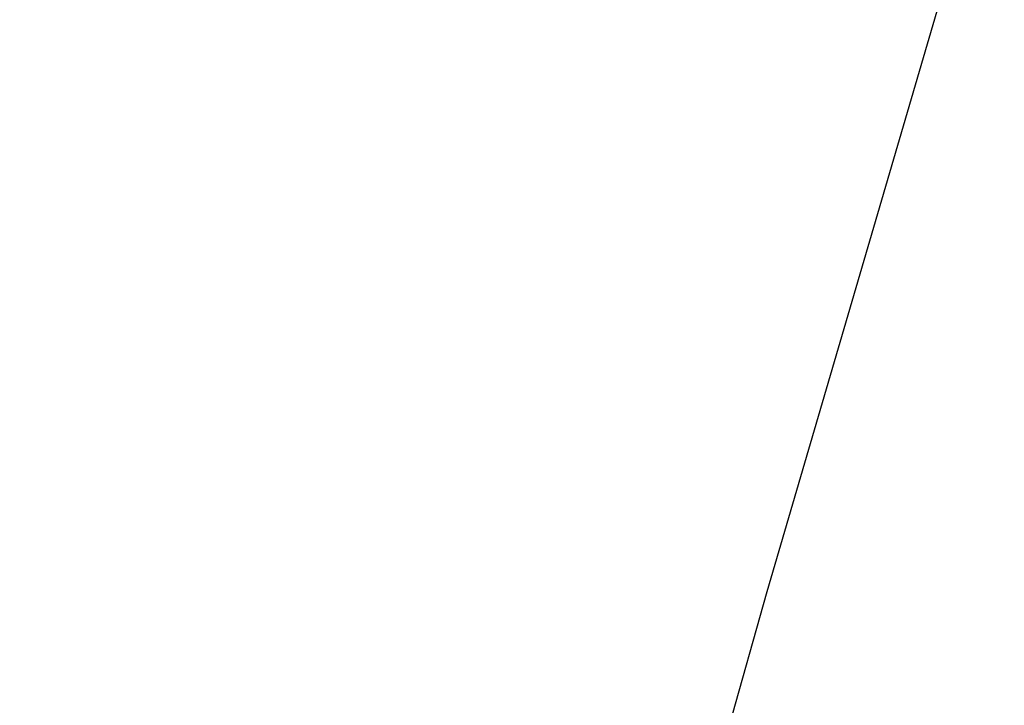
# Model space of a CAD drawing. Units: inches. Extents: x 3590 to 5167, y 65 to 1917.
# Tile 90 of 100: x 5052.5773 to 5052.8768, y 1788.6144 to 1788.8231. Entities that reach past the tile are written whole.
import ezdxf

# ---------------------------------------------------------------- set-up
doc = ezdxf.new("R2010")
doc.units = ezdxf.units.IN
for name, color, linetype, lineweight in [('A-ANNO-DIMS', 2, 'Continuous', 18), ('A-FLOR-PATT', 8, 'Continuous', 13), ('L-PLNT', 94, 'Continuous', 18)]:
    doc.layers.add(name, color=color, linetype=linetype, lineweight=lineweight)
doc.layers.add('DIENHOA', color=3, linetype='Continuous')
doc.styles.get("Standard").update_dxf_attribs({"font": 'arial.ttf'})
doc.dimstyles.new('ISO-25', dxfattribs={"dimtxt": 9, "dimasz": 2.5, "dimexe": 1.25, "dimexo": 0.625, "dimtad": 1, "dimdec": 1, "dimlunit": 3, "dimtxsty": 'Standard', "dimcen": 2.5, "dimadec": 0, "dimazin": 0, "dimtfac": 1, "dimtdec": 1, "dimtmove": 0, "dimatfit": 3, "dimfxl": 1, "dimarcsym": 0})

# ---------------------------------------------------------------- blocks, each defined once
blk = doc.blocks.new('Cay03_mb')
at = {"layer": 'DIENHOA'}
for p, q in [((118.956, 441.661), (96.72, 365.576)), ((96.72, 365.576), (75.598, 290.611))]:
    blk.add_line(p, q, dxfattribs=at)
blk = doc.blocks.new('*D323')
at = {"layer": 'A-ANNO-DIMS', "color": 0, "lineweight": -2, "transparency": 16777216}
for p, q in [((5069.17227, 1795.21603), (5069.17227, 1874.95034)), ((5065.43703, 1795.21603), (5070.42227, 1795.21603)), ((5069.17227, 1769.30924), (5069.17227, 1792.71603)), ((5065.43703, 1766.80924), (5070.42227, 1766.80924))]:
    blk.add_line(p, q, dxfattribs=at)
at = {"layer": 'A-ANNO-DIMS', "color": 0, "transparency": 16777216}
for points in [[(5068.75561, 1792.71603), (5069.58894, 1792.71603), (5069.17227, 1795.21603)], [(5068.75561, 1769.30924), (5069.58894, 1769.30924), (5069.17227, 1766.80924)]]:
    blk.add_solid(points, dxfattribs=at)
at = {"layer": 'Defpoints', "color": 0, "transparency": 16777216}
for p in [(5064.81203, 1795.21603), (5069.17227, 1795.21603), (5064.81203, 1766.80924)]:
    blk.add_point(p, dxfattribs=at)
at = {"layer": 'A-ANNO-DIMS', "color": 0, "transparency": 16777216, "insert": (5063.89379, 1836.33318), "char_height": 9, "attachment_point": 5, "rotation": 90}
blk.add_mtext('2\'-4 1/2" TYP.', dxfattribs=at)

msp = doc.modelspace()

# ---------------------------------------------------------------- hatches: boundary and pattern name
at = {"layer": 'A-FLOR-PATT', "transparency": 33554687}
h = msp.add_hatch(dxfattribs=at)
h.set_pattern_fill('AR-HBONE', color=256, scale=0.2)
h.set_pattern_definition([(45, (-588.972, 0), (0, 28.73682), [60.96, -20.32]), (135, (-574.604, 14.368), (3e-15, 28.73682), [60.96, -20.32])])
h.paths.add_polyline_path([(5071.27403, 1796.99898), (4933.27403, 1796.99898), (4933.27403, 1753.99898), (4962.77403, 1753.99898, -0.414214), (4928.77403, 1719.99898), (4933.27403, 1718.99898), (4933.27403, 1334.99898), (5071.27403, 1334.99898)])
h.paths.add_polyline_path([(4951.78002, 1521.0767), (4951.7151, 1521.0404), (4951.56345, 1520.89532)], flags=16)
h.paths.add_polyline_path([(4952.267, 1521.37645), (4952.1977, 1521.37111), (4952.19823, 1521.35558)], flags=0)
h.paths.add_polyline_path([(4967.05076, 1529.72832), (4965.23122, 1528.69444), (4963.41109, 1527.71401), (4961.75649, 1526.85081), (4963.58887, 1527.44938), (4964.03555, 1527.47802), (4962.9755, 1527.24902), (4961.76022, 1526.85203), (4959.79219, 1525.83406), (4958.00498, 1524.89483), (4956.24031, 1523.92961), (4954.50395, 1522.91854), (4954.1294, 1522.68163), (4953.36051, 1521.99688), (4953.36558, 1521.99754), (4953.605, 1522.06367), (4955.10605, 1522.76083), (4956.92108, 1523.43405), (4958.67784, 1523.91513), (4960.35834, 1524.20036), (4961.94456, 1524.28606), (4964.17144, 1524.10849), (4965.95752, 1523.30903), (4963.86273, 1522.97565), (4965.18742, 1522.49898), (4963.36614, 1522.49715), (4961.54526, 1522.48682), (4959.76359, 1522.46077), (4958.30414, 1522.4188), (4957.97356, 1522.38829), (4956.30692, 1522.2324), (4954.71821, 1522.07143), (4953.25077, 1521.89915), (4953.52509, 1521.62277), (4954.33087, 1521.37883), (4956.24263, 1521.22987), (4958.03913, 1520.92952), (4959.68424, 1520.48339), (4961.16007, 1519.89569), (4963.10699, 1518.80022), (4964.39286, 1517.32518), (4962.97306, 1517.72596), (4964.55841, 1516.66059), (4965.40664, 1515.70779), (4963.50733, 1516.32179), (4961.67995, 1517.0051), (4959.93478, 1517.74489), (4958.2821, 1518.52833), (4956.73216, 1519.34257), (4955.29527, 1520.17478), (4954.67155, 1520.57237), (4954.51279, 1520.6271), (4955.65848, 1519.31837), (4956.70263, 1517.98232), (4957.64403, 1516.64663), (4958.48545, 1515.33439), (4959.54998, 1513.52398), (4960.43768, 1511.76936), (4958.84107, 1513.6196), (4957.45175, 1515.3249), (4955.8186, 1517.45855), (4956.66537, 1515.44764), (4957.11109, 1513.92292), (4957.44681, 1511.71434), (4957.07641, 1509.79288), (4956.53757, 1511.1103), (4955.99231, 1512.56892), (4955.44448, 1514.12509), (4954.89794, 1515.73518), (4954.35653, 1517.35553), (4953.82412, 1518.94251), (4953.30455, 1520.45247), (4953.06452, 1521.11563), (4952.97143, 1521.14607), (4952.94932, 1521.08646), (4952.72981, 1520.19905), (4953.3698, 1518.02364), (4953.75708, 1516.37279), (4954.05124, 1514.76538), (4954.26449, 1513.22121), (4954.47124, 1511.13121), (4954.4971, 1510.40174), (4954.40903, 1511.76006), (4954.26449, 1513.22121), (4954.05124, 1514.76538), (4953.75708, 1516.37279), (4953.3698, 1518.02364), (4952.87718, 1519.69813), (4952.7161, 1520.1412), (4952.53301, 1519.05871), (4952.37428, 1517.78881), (4952.21925, 1516.31167), (4952.04598, 1514.59986), (4951.83253, 1512.62598), (4951.55697, 1510.36259), (4951.20331, 1512.16818), (4950.85168, 1514.33931), (4950.98529, 1516.37594), (4951.6596, 1518.28625), (4952.59261, 1520.48085), (4952.35664, 1521.1299), (4951.85502, 1520.32753), (4950.83901, 1518.90828), (4949.77675, 1517.58658), (4948.91554, 1516.61731), (4948.11099, 1515.2561), (4947.0891, 1513.55389), (4945.88937, 1511.61495), (4946.32587, 1513.40232), (4946.5624, 1514.24913), (4945.52771, 1513.32668), (4944.58105, 1512.53126), (4946.01774, 1514.50825), (4947.2044, 1516.04763), (4947.89331, 1517.31331), (4949.30686, 1518.76446), (4950.41417, 1519.76716), (4950.45131, 1519.80628), (4952.267, 1521.37645), (4951.64457, 1521.49317), (4950.40371, 1521.17954), (4948.04447, 1520.35868), (4946.11863, 1519.45198), (4944.57182, 1518.47484), (4943.34962, 1517.44265), (4941.99695, 1515.91971), (4941.66146, 1515.27475), (4942.81332, 1516.98973), (4944.57182, 1518.47484), (4946.11863, 1519.45198), (4948.04447, 1520.35868), (4950.40371, 1521.17954), (4951.64457, 1521.49317), (4949.64678, 1521.86781), (4948.59979, 1521.75633), (4947.12629, 1521.5699), (4945.42015, 1521.34763), (4943.44969, 1521.10462), (4941.18319, 1520.85596), (4942.86028, 1521.61265), (4943.87308, 1522.03014), (4942.95216, 1521.9093), (4941.40968, 1521.48512), (4939.54287, 1520.67019), (4938.96775, 1520.2255), (4940.73284, 1521.29899), (4942.95216, 1521.9093), (4943.70184, 1522.00767), (4945.89419, 1522.69998), (4947.56488, 1522.71399), (4948.92086, 1522.56573), (4951.13144, 1522.18271), (4950.97062, 1522.2969), (4948.12924, 1523.00563), (4946.03496, 1523.70671), (4944.23235, 1524.52143), (4942.70692, 1525.46111), (4941.44419, 1526.53707), (4940.42968, 1527.76062), (4939.6489, 1529.14306), (4941.42091, 1528.12232), (4943.14742, 1527.13248), (4944.84093, 1526.17457), (4946.51394, 1525.24959), (4948.17893, 1524.35855), (4948.36457, 1524.26336), (4946.47531, 1526.04459), (4945.18083, 1527.54042), (4944.19039, 1529.03339), (4943.49559, 1530.53985), (4943.27808, 1531.3597), (4942.49849, 1531.91903), (4943.11353, 1531.76249), (4942.95927, 1533.6586), (4944.13953, 1531.9886), (4944.61171, 1531.32339), (4946.20163, 1530.46341), (4947.48567, 1529.50925), (4948.79027, 1528.22649), (4950.36754, 1526.23746), (4949.48547, 1528.15549), (4948.85128, 1530.12254), (4948.49054, 1532.04127), (4948.38105, 1533.91822), (4948.50062, 1535.7599), (4948.82704, 1537.57284), (4949.41803, 1535.56526), (4949.95684, 1533.56932), (4950.46414, 1531.5861), (4950.96058, 1529.6167), (4951.3911, 1527.95448), (4951.72352, 1530.68689), (4952.20106, 1532.57994), (4952.88914, 1534.32964), (4953.77035, 1535.95123), (4954.82726, 1537.45995), (4954.52145, 1535.38966), (4954.27314, 1533.93684), (4955.57999, 1535.6627), (4956.74758, 1536.73859), (4956.15852, 1534.78029), (4955.58917, 1532.87334), (4955.04336, 1531.00581), (4954.52493, 1529.16576), (4954.03771, 1527.34127), (4953.63833, 1525.73298), (4953.61143, 1525.58564), (4953.39805, 1524.16565), (4953.38219, 1524.00887), (4954.06955, 1525.47563), (4954.91212, 1527.02173), (4956.13627, 1528.89351), (4957.84668, 1530.57701), (4959.37601, 1531.54014), (4958.25596, 1530.10398), (4957.14284, 1528.66291), (4956.06626, 1527.24305), (4955.05579, 1525.87054), (4954.14104, 1524.57149), (4953.35159, 1523.37204), (4953.31079, 1523.30299), (4953.27253, 1522.92478), (4953.26102, 1522.38213), (4954.1031, 1523.37273), (4954.63005, 1524.28376), (4955.96149, 1526.35767), (4957.23002, 1528.12969), (4958.42057, 1529.60864), (4960.03671, 1531.36792), (4961.3736, 1532.3752), (4962.1015, 1532.77), (4961.06994, 1531.06113), (4959.98733, 1529.43811), (4958.86851, 1527.90803), (4958.15046, 1527.00742), (4959.80291, 1528.00314), (4961.58854, 1528.79257), (4963.39087, 1529.32783), (4965.21118, 1529.63205)], flags=16)
h.paths.add_polyline_path([(4962.94387, 1523.18187), (4961.10714, 1523.42192), (4960.39205, 1523.36158), (4962.34964, 1523.33061)], flags=0)
h.paths.add_polyline_path([(5049.54129, 1584.55089), (5049.47636, 1584.51458), (5049.32471, 1584.3695)], flags=16)
h.paths.add_polyline_path([(5050.02827, 1584.85063), (5049.95897, 1584.84529), (5049.95949, 1584.82976)], flags=0)
h.paths.add_polyline_path([(5042.33308, 1581.94902), (5043.8799, 1582.92616), (5045.80573, 1583.83286), (5048.16498, 1584.65372), (5049.40583, 1584.96736), (5047.40804, 1585.34199), (5046.36106, 1585.23052), (5044.88755, 1585.04408), (5043.18142, 1584.82181), (5041.21095, 1584.5788), (5038.94446, 1584.33014), (5040.62155, 1585.08683), (5041.63434, 1585.50432), (5040.71343, 1585.38348), (5039.17095, 1584.9593), (5037.30414, 1584.14438), (5036.72901, 1583.69969), (5038.4941, 1584.77317), (5040.71343, 1585.38348), (5041.4631, 1585.48185), (5043.65545, 1586.17416), (5045.32615, 1586.18818), (5046.68212, 1586.03992), (5048.8927, 1585.6569), (5048.73188, 1585.77108), (5045.89051, 1586.47981), (5043.79622, 1587.18089), (5041.99361, 1587.99561), (5040.46818, 1588.9353), (5039.20546, 1590.01125), (5038.19095, 1591.2348), (5037.41016, 1592.61725), (5039.18217, 1591.5965), (5040.90868, 1590.60667), (5042.6022, 1589.64876), (5044.2752, 1588.72378), (5045.94019, 1587.83274), (5046.12584, 1587.73754), (5044.23658, 1589.51878), (5042.9421, 1591.01461), (5041.95166, 1592.50757), (5041.25685, 1594.01403), (5041.03935, 1594.83388), (5040.25976, 1595.39321), (5040.8748, 1595.23667), (5040.72054, 1597.13279), (5041.9008, 1595.46278), (5042.37297, 1594.79758), (5043.96289, 1593.93759), (5045.24694, 1592.98344), (5046.55153, 1591.70068), (5048.12881, 1589.71164), (5047.24673, 1591.62967), (5046.61254, 1593.59672), (5046.2518, 1595.51546), (5046.14232, 1597.3924), (5046.26189, 1599.23408), (5046.5883, 1601.04703), (5047.17929, 1599.03944), (5047.71811, 1597.0435), (5048.22541, 1595.06028), (5048.72184, 1593.09089), (5049.15237, 1591.42866), (5049.48478, 1594.16107), (5049.96233, 1596.05412), (5050.65041, 1597.80382), (5051.53161, 1599.42541), (5052.58852, 1600.93414), (5052.28271, 1598.86384), (5052.03441, 1597.41102), (5053.34126, 1599.13689), (5054.50884, 1600.21277), (5053.91979, 1598.25447), (5053.35044, 1596.34752), (5052.80463, 1594.47999), (5052.2862, 1592.63995), (5051.79898, 1590.81546), (5051.39959, 1589.20716), (5051.3727, 1589.05983), (5051.15931, 1587.63984), (5051.14346, 1587.48305), (5051.83082, 1588.94982), (5052.67339, 1590.49592), (5053.89754, 1592.3677), (5055.60794, 1594.05119), (5057.13728, 1595.01432), (5056.01722, 1593.57817), (5054.90411, 1592.1371), (5053.82752, 1590.71724), (5052.81705, 1589.34472), (5051.9023, 1588.04567), (5051.11286, 1586.84622), (5051.07205, 1586.77718), (5051.03379, 1586.39896), (5051.02228, 1585.85631), (5051.86437, 1586.84692), (5052.39131, 1587.75794), (5053.72275, 1589.83185), (5054.99128, 1591.60387), (5056.18183, 1593.08282), (5057.79798, 1594.84211), (5059.13486, 1595.84938), (5059.86276, 1596.24419), (5058.83121, 1594.53531), (5057.7486, 1592.9123), (5056.62978, 1591.38221), (5055.91173, 1590.4816), (5057.56418, 1591.47732), (5059.34981, 1592.26675), (5061.15214, 1592.80202), (5062.97245, 1593.10624), (5064.81203, 1593.20251), (5062.99248, 1592.16863), (5061.17235, 1591.18819), (5059.51775, 1590.325), (5061.35014, 1590.92356), (5061.79682, 1590.95221), (5060.73676, 1590.7232), (5059.52148, 1590.32622), (5057.55345, 1589.30825), (5055.76625, 1588.36901), (5054.00157, 1587.40379), (5052.26521, 1586.39273), (5051.89067, 1586.15581), (5051.12177, 1585.47106), (5051.12684, 1585.47172), (5051.36627, 1585.53786), (5052.86732, 1586.23502), (5054.68234, 1586.90824), (5056.4391, 1587.38931), (5058.1196, 1587.67454), (5059.70582, 1587.76024), (5061.93271, 1587.58268), (5063.71878, 1586.78321), (5061.62399, 1586.44983), (5062.94869, 1585.97317), (5061.12741, 1585.97133), (5059.30653, 1585.961), (5057.52486, 1585.93496), (5056.06541, 1585.89299), (5055.73482, 1585.86247), (5054.06819, 1585.70658), (5052.47947, 1585.54561), (5051.01204, 1585.37333), (5051.28635, 1585.09695), (5052.09214, 1584.85301), (5054.00389, 1584.70406), (5055.8004, 1584.4037), (5057.44551, 1583.95757), (5058.92133, 1583.36987), (5060.86825, 1582.27441), (5062.15413, 1580.79937), (5060.73433, 1581.20015), (5062.31967, 1580.13477), (5063.1679, 1579.18198), (5061.2686, 1579.79597), (5059.44122, 1580.47928), (5057.69605, 1581.21908), (5056.04336, 1582.00251), (5054.49343, 1582.81675), (5053.05653, 1583.64897), (5052.43281, 1584.04656), (5052.27405, 1584.10128), (5053.41974, 1582.79255), (5054.4639, 1581.4565), (5055.40529, 1580.12081), (5056.24672, 1578.80858), (5057.31125, 1576.99816), (5058.19895, 1575.24354), (5056.60234, 1577.09378), (5055.21301, 1578.79908), (5053.57987, 1580.93274), (5054.42664, 1578.92183), (5054.87235, 1577.3971), (5055.20808, 1575.18852), (5054.83767, 1573.26706), (5054.29883, 1574.58448), (5053.75357, 1576.0431), (5053.20575, 1577.59927), (5052.6592, 1579.20936), (5052.1178, 1580.82971), (5051.58538, 1582.41669), (5051.06582, 1583.92666), (5050.82578, 1584.58981), (5050.7327, 1584.62025), (5050.71058, 1584.56064), (5050.49108, 1583.67323), (5051.13107, 1581.49782), (5051.51835, 1579.84698), (5051.8125, 1578.23957), (5052.02575, 1576.69539), (5052.23251, 1574.6054), (5052.25836, 1573.87593), (5052.1703, 1575.23424), (5052.02575, 1576.69539), (5051.8125, 1578.23957), (5051.51835, 1579.84698), (5051.13107, 1581.49782), (5050.63844, 1583.17231), (5050.47736, 1583.61538), (5050.29428, 1582.53289), (5050.13554, 1581.26299), (5049.98051, 1579.78585), (5049.80724, 1578.07405), (5049.59379, 1576.10016), (5049.31823, 1573.83678), (5048.96458, 1575.64237), (5048.61294, 1577.8135), (5048.74656, 1579.85012), (5049.42086, 1581.76043), (5050.35388, 1583.95503), (5050.1179, 1584.60408), (5049.61629, 1583.80172), (5048.60027, 1582.38246), (5047.53801, 1581.06076), (5046.67681, 1580.09149), (5045.87225, 1578.73029), (5044.85036, 1577.02808), (5043.65063, 1575.08913), (5044.08713, 1576.8765), (5044.32366, 1577.72331), (5043.28898, 1576.80086), (5042.34232, 1576.00545), (5043.779, 1577.98243), (5044.96566, 1579.52182), (5045.65457, 1580.78749), (5047.06813, 1582.23865), (5048.17543, 1583.24134), (5048.21258, 1583.28047), (5050.02827, 1584.85063), (5049.40583, 1584.96736), (5048.16498, 1584.65372), (5045.80573, 1583.83286), (5043.8799, 1582.92616), (5042.33308, 1581.94902), (5041.11088, 1580.91684), (5039.75821, 1579.39389), (5039.42272, 1578.74894), (5040.57458, 1580.46391)], flags=16)
h.paths.add_polyline_path([(4954.79872, 1533.12029), (4954.26249, 1532.07935), (4953.83112, 1530.93464), (4953.50472, 1529.63602), (4953.28338, 1528.13331), (4953.16721, 1526.37637), (4953.15631, 1524.31504), (4953.27669, 1521.23629), (4952.80168, 1521.84177), (4951.55695, 1521.99789), (4950.97575, 1521.9613), (4952.66059, 1521.94097), (4952.80168, 1521.84177), (4953.15249, 1523.59258), (4953.16721, 1526.37637), (4953.28338, 1528.13331), (4953.60929, 1530.34598), (4954.45558, 1532.59174)], flags=0)
h.paths.add_polyline_path([(5050.56294, 1585.31596), (5049.31822, 1585.47208), (5048.73702, 1585.43548), (5050.42186, 1585.41516), (5050.56294, 1585.31596), (5050.91375, 1587.06676), (5050.92848, 1589.85056), (5051.04465, 1591.6075), (5051.37055, 1593.82017), (5052.21684, 1596.06593), (5052.55999, 1596.59447), (5052.02375, 1595.55353), (5051.59238, 1594.40883), (5051.26598, 1593.1102), (5051.04465, 1591.6075), (5050.92848, 1589.85056), (5050.91757, 1587.78922), (5051.03795, 1584.71048)], flags=0)
h.paths.add_polyline_path([(5058.15332, 1586.83576), (5060.11091, 1586.80479), (5060.70514, 1586.65605), (5058.8684, 1586.8961)], flags=0)
h.paths.add_polyline_path([(5049.54129, 1430.93611), (5049.47636, 1430.8998), (5049.32471, 1430.75472)], flags=16)
h.paths.add_polyline_path([(5050.02827, 1431.23585), (5049.95897, 1431.23051), (5049.95949, 1431.21498)], flags=0)
h.paths.add_polyline_path([(5046.5883, 1447.43225), (5047.17929, 1445.42467), (5047.71811, 1443.42872), (5048.22541, 1441.4455), (5048.72184, 1439.47611), (5049.15237, 1437.81388), (5049.48478, 1440.5463), (5049.96233, 1442.43934), (5050.65041, 1444.18904), (5051.53161, 1445.81063), (5052.58852, 1447.31936), (5052.28271, 1445.24906), (5052.03441, 1443.79624), (5053.34126, 1445.52211), (5054.50884, 1446.59799), (5053.91979, 1444.63969), (5053.35044, 1442.73274), (5052.80463, 1440.86521), (5052.2862, 1439.02517), (5051.79898, 1437.20068), (5051.39959, 1435.59238), (5051.3727, 1435.44505), (5051.15931, 1434.02506), (5051.14346, 1433.86828), (5051.83082, 1435.33504), (5052.67339, 1436.88114), (5053.89754, 1438.75292), (5055.60794, 1440.43641), (5057.13728, 1441.39954), (5056.01722, 1439.96339), (5054.90411, 1438.52232), (5053.82752, 1437.10246), (5052.81705, 1435.72994), (5051.9023, 1434.4309), (5051.11286, 1433.23145), (5051.07205, 1433.1624), (5051.03379, 1432.78418), (5051.02228, 1432.24153), (5051.86437, 1433.23214), (5052.39131, 1434.14316), (5053.72275, 1436.21707), (5054.99128, 1437.98909), (5056.18183, 1439.46805), (5057.79798, 1441.22733), (5059.13486, 1442.23461), (5059.86276, 1442.62941), (5058.83121, 1440.92053), (5057.7486, 1439.29752), (5056.62978, 1437.76743), (5055.91173, 1436.86682), (5057.56418, 1437.86255), (5059.34981, 1438.65197), (5061.15214, 1439.18724), (5062.97245, 1439.49146), (5064.81203, 1439.58773), (5062.99248, 1438.55385), (5061.17235, 1437.57342), (5059.51775, 1436.71022), (5061.35014, 1437.30879), (5061.79682, 1437.33743), (5060.73676, 1437.10842), (5059.52148, 1436.71144), (5057.55345, 1435.69347), (5055.76625, 1434.75423), (5054.00157, 1433.78901), (5052.26521, 1432.77795), (5051.89067, 1432.54103), (5051.12177, 1431.85628), (5051.12684, 1431.85694), (5051.36627, 1431.92308), (5052.86732, 1432.62024), (5054.68234, 1433.29346), (5056.4391, 1433.77453), (5058.1196, 1434.05976), (5059.70582, 1434.14546), (5061.93271, 1433.9679), (5063.71878, 1433.16843), (5061.62399, 1432.83505), (5062.94869, 1432.35839), (5061.12741, 1432.35655), (5059.30653, 1432.34623), (5057.52486, 1432.32018), (5056.06541, 1432.27821), (5055.73482, 1432.24769), (5054.06819, 1432.09181), (5052.47947, 1431.93083), (5051.01204, 1431.75856), (5051.28635, 1431.48218), (5052.09214, 1431.23823), (5054.00389, 1431.08928), (5055.8004, 1430.78892), (5057.44551, 1430.34279), (5058.92133, 1429.75509), (5060.86825, 1428.65963), (5062.15413, 1427.18459), (5060.73433, 1427.58537), (5062.31967, 1426.52), (5063.1679, 1425.5672), (5061.2686, 1426.18119), (5059.44122, 1426.86451), (5057.69605, 1427.6043), (5056.04336, 1428.38773), (5054.49343, 1429.20197), (5053.05653, 1430.03419), (5052.43281, 1430.43178), (5052.27405, 1430.48651), (5053.41974, 1429.17777), (5054.4639, 1427.84172), (5055.40529, 1426.50603), (5056.24672, 1425.1938), (5057.31125, 1423.38338), (5058.19895, 1421.62877), (5056.60234, 1423.479), (5055.21301, 1425.1843), (5053.57987, 1427.31796), (5054.42664, 1425.30705), (5054.87235, 1423.78233), (5055.20808, 1421.57374), (5054.83767, 1419.65228), (5054.29883, 1420.9697), (5053.75357, 1422.42832), (5053.20575, 1423.9845), (5052.6592, 1425.59458), (5052.1178, 1427.21493), (5051.58538, 1428.80191), (5051.06582, 1430.31188), (5050.82578, 1430.97503), (5050.7327, 1431.00547), (5050.71058, 1430.94586), (5050.49108, 1430.05845), (5051.13107, 1427.88305), (5051.51835, 1426.2322), (5051.8125, 1424.62479), (5052.02575, 1423.08061), (5052.23251, 1420.99062), (5052.25836, 1420.26115), (5052.1703, 1421.61947), (5052.02575, 1423.08061), (5051.8125, 1424.62479), (5051.51835, 1426.2322), (5051.13107, 1427.88305), (5050.63844, 1429.55753), (5050.47736, 1430.0006), (5050.29428, 1428.91811), (5050.13554, 1427.64821), (5049.98051, 1426.17107), (5049.80724, 1424.45927), (5049.59379, 1422.48539), (5049.31823, 1420.222), (5048.96458, 1422.02759), (5048.61294, 1424.19872), (5048.74656, 1426.23534), (5049.42086, 1428.14565), (5050.35388, 1430.34025), (5050.1179, 1430.98931), (5049.61629, 1430.18694), (5048.60027, 1428.76768), (5047.53801, 1427.44598), (5046.67681, 1426.47671), (5045.87225, 1425.11551), (5044.85036, 1423.4133), (5043.65063, 1421.47435), (5044.08713, 1423.26172), (5044.32366, 1424.10854), (5043.28898, 1423.18608), (5042.34232, 1422.39067), (5043.779, 1424.36765), (5044.96566, 1425.90704), (5045.65457, 1427.17272), (5047.06813, 1428.62387), (5048.17543, 1429.62657), (5048.21258, 1429.66569), (5050.02827, 1431.23585), (5049.40583, 1431.35258), (5048.16498, 1431.03894), (5045.80573, 1430.21809), (5043.8799, 1429.31139), (5042.33308, 1428.33424), (5041.11088, 1427.30206), (5039.75821, 1425.77911), (5039.42272, 1425.13416), (5040.57458, 1426.84914), (5042.33308, 1428.33424), (5043.8799, 1429.31139), (5045.80573, 1430.21809), (5048.16498, 1431.03894), (5049.40583, 1431.35258), (5047.40804, 1431.72722), (5046.36106, 1431.61574), (5044.88755, 1431.42931), (5043.18142, 1431.20704), (5041.21095, 1430.96402), (5038.94446, 1430.71536), (5040.62155, 1431.47205), (5041.63434, 1431.88954), (5040.71343, 1431.76871), (5039.17095, 1431.34453), (5037.30414, 1430.5296), (5036.72901, 1430.08491), (5038.4941, 1431.1584), (5040.71343, 1431.76871), (5041.4631, 1431.86707), (5043.65545, 1432.55939), (5045.32615, 1432.5734), (5046.68212, 1432.42514), (5048.8927, 1432.04212), (5048.73188, 1432.1563), (5045.89051, 1432.86503), (5043.79622, 1433.56611), (5041.99361, 1434.38083), (5040.46818, 1435.32052), (5039.20546, 1436.39648), (5038.19095, 1437.62002), (5037.41016, 1439.00247), (5039.18217, 1437.98172), (5040.90868, 1436.99189), (5042.6022, 1436.03398), (5044.2752, 1435.109), (5045.94019, 1434.21796), (5046.12584, 1434.12276), (5044.23658, 1435.904), (5042.9421, 1437.39983), (5041.95166, 1438.8928), (5041.25685, 1440.39925), (5041.03935, 1441.2191), (5040.25976, 1441.77844), (5040.8748, 1441.62189), (5040.72054, 1443.51801), (5041.9008, 1441.848), (5042.37297, 1441.1828), (5043.96289, 1440.32282), (5045.24694, 1439.36866), (5046.55153, 1438.0859), (5048.12881, 1436.09686), (5047.24673, 1438.01489), (5046.61254, 1439.98195), (5046.2518, 1441.90068), (5046.14232, 1443.77762), (5046.26189, 1445.6193)], flags=16)
h.paths.add_polyline_path([(5052.38176, 1444.25496), (5051.62263, 1442.77987), (5052.02375, 1441.93875), (5052.55999, 1442.9797)], flags=0)
h.paths.add_polyline_path([(5050.56294, 1431.70118), (5049.31822, 1431.8573), (5048.73702, 1431.82071), (5050.42186, 1431.80038)], flags=0)
h.paths.add_polyline_path([(5058.15332, 1433.22098), (5060.11091, 1433.19001), (5060.70514, 1433.04127), (5058.8684, 1433.28132)], flags=0)
h.paths.add_polyline_path([(5049.54129, 1352.28535), (5049.47636, 1352.24904), (5049.32471, 1352.10396)], flags=16)
h.paths.add_polyline_path([(5050.02827, 1352.58509), (5049.95897, 1352.57975), (5049.95949, 1352.56422)], flags=0)
h.paths.add_polyline_path([(5046.5883, 1368.78149), (5047.17929, 1366.7739), (5047.71811, 1364.77796), (5048.22541, 1362.79474), (5048.72184, 1360.82534), (5049.15237, 1359.16312), (5049.48478, 1361.89553), (5049.96233, 1363.78858), (5050.65041, 1365.53828), (5051.53161, 1367.15987), (5052.58852, 1368.6686), (5052.28271, 1366.5983), (5052.03441, 1365.14548), (5053.34126, 1366.87135), (5054.50884, 1367.94723), (5053.91979, 1365.98893), (5053.35044, 1364.08198), (5052.80463, 1362.21445), (5052.2862, 1360.37441), (5051.79898, 1358.54992), (5051.39959, 1356.94162), (5051.3727, 1356.79428), (5051.15931, 1355.37429), (5051.14346, 1355.21751), (5051.83082, 1356.68428), (5052.67339, 1358.23037), (5053.89754, 1360.10216), (5055.60794, 1361.78565), (5057.13728, 1362.74878), (5056.01722, 1361.31262), (5054.90411, 1359.87155), (5053.82752, 1358.4517), (5052.81705, 1357.07918), (5051.9023, 1355.78013), (5051.11286, 1354.58068), (5051.07205, 1354.51164), (5051.03379, 1354.13342), (5051.02228, 1353.59077), (5051.86437, 1354.58137), (5052.39131, 1355.4924), (5053.72275, 1357.56631), (5054.99128, 1359.33833), (5056.18183, 1360.81728), (5057.79798, 1362.57656), (5059.13486, 1363.58384), (5059.86276, 1363.97864), (5058.83121, 1362.26977), (5057.7486, 1360.64675), (5056.62978, 1359.11667), (5055.91173, 1358.21606), (5057.56418, 1359.21178), (5059.34981, 1360.00121), (5061.15214, 1360.53648), (5062.97245, 1360.84069), (5064.81203, 1360.93697), (5062.99248, 1359.90308), (5061.17235, 1358.92265), (5059.51775, 1358.05946), (5061.35014, 1358.65802), (5061.79682, 1358.68666), (5060.73676, 1358.45766), (5059.52148, 1358.06068), (5057.55345, 1357.0427), (5055.76625, 1356.10347), (5054.00157, 1355.13825), (5052.26521, 1354.12718), (5051.89067, 1353.89027), (5051.12177, 1353.20552), (5051.12684, 1353.20618), (5051.36627, 1353.27231), (5052.86732, 1353.96947), (5054.68234, 1354.6427), (5056.4391, 1355.12377), (5058.1196, 1355.409), (5059.70582, 1355.4947), (5061.93271, 1355.31713), (5063.71878, 1354.51767), (5061.62399, 1354.18429), (5062.94869, 1353.70763), (5061.12741, 1353.70579), (5059.30653, 1353.69546), (5057.52486, 1353.66942), (5056.06541, 1353.62744), (5055.73482, 1353.59693), (5054.06819, 1353.44104), (5052.47947, 1353.28007), (5051.01204, 1353.10779), (5051.28635, 1352.83141), (5052.09214, 1352.58747), (5054.00389, 1352.43852), (5055.8004, 1352.13816), (5057.44551, 1351.69203), (5058.92133, 1351.10433), (5060.86825, 1350.00887), (5062.15413, 1348.53382), (5060.73433, 1348.9346), (5062.31967, 1347.86923), (5063.1679, 1346.91643), (5061.2686, 1347.53043), (5059.44122, 1348.21374), (5057.69605, 1348.95353), (5056.04336, 1349.73697), (5054.49343, 1350.55121), (5053.05653, 1351.38342), (5052.43281, 1351.78101), (5052.27405, 1351.83574), (5053.41974, 1350.52701), (5054.4639, 1349.19096), (5055.40529, 1347.85527), (5056.24672, 1346.54303), (5057.31125, 1344.73262), (5058.19895, 1342.978), (5056.60234, 1344.82824), (5055.21301, 1346.53354), (5053.57987, 1348.6672), (5054.42664, 1346.65629), (5054.87235, 1345.13156), (5055.20808, 1342.92298), (5054.83767, 1341.00152), (5054.29883, 1342.31894), (5053.75357, 1343.77756), (5053.20575, 1345.33373), (5052.6592, 1346.94382), (5052.1178, 1348.56417), (5051.58538, 1350.15115), (5051.06582, 1351.66111), (5050.82578, 1352.32427), (5050.7327, 1352.35471), (5050.71058, 1352.2951), (5050.49108, 1351.40769), (5051.13107, 1349.23228), (5051.51835, 1347.58144), (5051.8125, 1345.97403), (5052.02575, 1344.42985), (5052.23251, 1342.33986), (5052.25836, 1341.61039), (5052.1703, 1342.9687), (5052.02575, 1344.42985), (5051.8125, 1345.97403), (5051.51835, 1347.58144), (5051.13107, 1349.23228), (5050.63844, 1350.90677), (5050.47736, 1351.34984), (5050.29428, 1350.26735), (5050.13554, 1348.99745), (5049.98051, 1347.52031), (5049.80724, 1345.80851), (5049.59379, 1343.83462), (5049.31823, 1341.57124), (5048.96458, 1343.37683), (5048.61294, 1345.54796), (5048.74656, 1347.58458), (5049.42086, 1349.49489), (5050.35388, 1351.68949), (5050.1179, 1352.33854), (5049.61629, 1351.53617), (5048.60027, 1350.11692), (5047.53801, 1348.79522), (5046.67681, 1347.82595), (5045.87225, 1346.46475), (5044.85036, 1344.76253), (5043.65063, 1342.82359), (5044.08713, 1344.61096), (5044.32366, 1345.45777), (5043.28898, 1344.53532), (5042.34232, 1343.7399), (5043.779, 1345.71689), (5044.96566, 1347.25627), (5045.65457, 1348.52195), (5047.06813, 1349.9731), (5048.17543, 1350.9758), (5048.21258, 1351.01493), (5050.02827, 1352.58509), (5049.40583, 1352.70181), (5048.16498, 1352.38818), (5045.80573, 1351.56732), (5043.8799, 1350.66062), (5042.33308, 1349.68348), (5041.11088, 1348.65129), (5039.75821, 1347.12835), (5039.42272, 1346.4834), (5040.57458, 1348.19837), (5042.33308, 1349.68348), (5043.8799, 1350.66062), (5045.80573, 1351.56732), (5048.16498, 1352.38818), (5049.40583, 1352.70181), (5047.40804, 1353.07645), (5046.36106, 1352.96498), (5044.88755, 1352.77854), (5043.18142, 1352.55627), (5041.21095, 1352.31326), (5038.94446, 1352.0646), (5040.62155, 1352.82129), (5041.63434, 1353.23878), (5040.71343, 1353.11794), (5039.17095, 1352.69376), (5037.30414, 1351.87884), (5036.72901, 1351.43415), (5038.4941, 1352.50763), (5040.71343, 1353.11794), (5041.4631, 1353.21631), (5043.65545, 1353.90862), (5045.32615, 1353.92263), (5046.68212, 1353.77438), (5048.8927, 1353.39136), (5048.73188, 1353.50554), (5045.89051, 1354.21427), (5043.79622, 1354.91535), (5041.99361, 1355.73007), (5040.46818, 1356.66975), (5039.20546, 1357.74571), (5038.19095, 1358.96926), (5037.41016, 1360.35171), (5039.18217, 1359.33096), (5040.90868, 1358.34112), (5042.6022, 1357.38321), (5044.2752, 1356.45824), (5045.94019, 1355.5672), (5046.12584, 1355.472), (5044.23658, 1357.25323), (5042.9421, 1358.74906), (5041.95166, 1360.24203), (5041.25685, 1361.74849), (5041.03935, 1362.56834), (5040.25976, 1363.12767), (5040.8748, 1362.97113), (5040.72054, 1364.86725), (5041.9008, 1363.19724), (5042.37297, 1362.53203), (5043.96289, 1361.67205), (5045.24694, 1360.7179), (5046.55153, 1359.43513), (5048.12881, 1357.4461), (5047.24673, 1359.36413), (5046.61254, 1361.33118), (5046.2518, 1363.24992), (5046.14232, 1365.12686), (5046.26189, 1366.96854)], flags=16)
h.paths.add_polyline_path([(5052.38176, 1365.6042), (5051.62263, 1364.12911), (5052.02375, 1363.28799), (5052.55999, 1364.32893)], flags=0)
h.paths.add_polyline_path([(4951.78002, 1698.04081), (4951.7151, 1698.0045), (4951.56345, 1697.85942)], flags=16)
h.paths.add_polyline_path([(4952.267, 1698.34055), (4952.1977, 1698.33521), (4952.19823, 1698.31968)], flags=0)
h.paths.add_polyline_path([(4957.07641, 1686.75698), (4956.53757, 1688.0744), (4955.99231, 1689.53302), (4955.44448, 1691.08919), (4954.89794, 1692.69928), (4954.35653, 1694.31963), (4953.82412, 1695.90661), (4953.30455, 1697.41658), (4953.06452, 1698.07973), (4952.97143, 1698.11017), (4952.94932, 1698.05056), (4952.72981, 1697.16315), (4953.3698, 1694.98774), (4953.75708, 1693.3369), (4954.05124, 1691.72949), (4954.26449, 1690.18531), (4954.47124, 1688.09532), (4954.4971, 1687.36585), (4954.40903, 1688.72416), (4954.26449, 1690.18531), (4954.05124, 1691.72949), (4953.75708, 1693.3369), (4953.3698, 1694.98774), (4952.87718, 1696.66223), (4952.7161, 1697.1053), (4952.53301, 1696.02281), (4952.37428, 1694.75291), (4952.21925, 1693.27577), (4952.04598, 1691.56397), (4951.83253, 1689.59008), (4951.55697, 1687.3267), (4951.20331, 1689.13229), (4950.85168, 1691.30342), (4950.98529, 1693.34004), (4951.6596, 1695.25035), (4952.59261, 1697.44495), (4952.35664, 1698.09401), (4951.85502, 1697.29164), (4950.83901, 1695.87238), (4949.77675, 1694.55068), (4948.91554, 1693.58141), (4948.11099, 1692.22021), (4947.0891, 1690.518), (4945.88937, 1688.57905), (4946.32587, 1690.36642), (4946.5624, 1691.21323), (4945.52771, 1690.29078), (4944.58105, 1689.49537), (4946.01774, 1691.47235), (4947.2044, 1693.01174), (4947.89331, 1694.27741), (4949.30686, 1695.72857), (4950.41417, 1696.73127), (4950.45131, 1696.77039), (4952.267, 1698.34055), (4951.64457, 1698.45728), (4950.40371, 1698.14364), (4948.04447, 1697.32278), (4946.11863, 1696.41608), (4944.57182, 1695.43894), (4943.34962, 1694.40676), (4941.99695, 1692.88381), (4941.66146, 1692.23886), (4942.81332, 1693.95383), (4944.57182, 1695.43894), (4946.11863, 1696.41608), (4948.04447, 1697.32278), (4950.40371, 1698.14364), (4951.64457, 1698.45728), (4949.64678, 1698.83191), (4948.59979, 1698.72044), (4947.12629, 1698.53401), (4945.42015, 1698.31174), (4943.44969, 1698.06872), (4941.18319, 1697.82006), (4942.86028, 1698.57675), (4943.87308, 1698.99424), (4942.95216, 1698.8734), (4941.40968, 1698.44922), (4939.54287, 1697.6343), (4938.96775, 1697.18961), (4940.73284, 1698.26309), (4942.95216, 1698.8734), (4943.70184, 1698.97177), (4945.89419, 1699.66409), (4947.56488, 1699.6781), (4948.92086, 1699.52984), (4951.13144, 1699.14682), (4950.97062, 1699.261), (4948.12924, 1699.96973), (4946.03496, 1700.67081), (4944.23235, 1701.48553), (4942.70692, 1702.42522), (4941.44419, 1703.50117), (4940.42968, 1704.72472), (4939.6489, 1706.10717), (4941.42091, 1705.08642), (4943.14742, 1704.09659), (4944.84093, 1703.13868), (4946.51394, 1702.2137), (4948.17893, 1701.32266), (4948.36457, 1701.22746), (4946.47531, 1703.0087), (4945.18083, 1704.50453), (4944.19039, 1705.9975), (4943.49559, 1707.50395), (4943.27808, 1708.3238), (4942.49849, 1708.88314), (4943.11353, 1708.72659), (4942.95927, 1710.62271), (4944.13953, 1708.9527), (4944.61171, 1708.2875), (4946.20163, 1707.42751), (4947.48567, 1706.47336), (4948.79027, 1705.1906), (4950.36754, 1703.20156), (4949.48547, 1705.11959), (4948.85128, 1707.08664), (4948.49054, 1709.00538), (4948.38105, 1710.88232), (4948.50062, 1712.724), (4948.82704, 1714.53695), (4949.41803, 1712.52937), (4949.95684, 1710.53342), (4950.46414, 1708.5502), (4950.96058, 1706.58081), (4951.3911, 1704.91858), (4951.72352, 1707.65099), (4952.20106, 1709.54404), (4952.88914, 1711.29374), (4953.77035, 1712.91533), (4954.82726, 1714.42406), (4954.52145, 1712.35376), (4954.27314, 1710.90094), (4955.57999, 1712.62681), (4956.74758, 1713.70269), (4956.15852, 1711.74439), (4955.58917, 1709.83744), (4955.04336, 1707.96991), (4954.52493, 1706.12987), (4954.03771, 1704.30538), (4953.63833, 1702.69708), (4953.61143, 1702.54975), (4953.39805, 1701.12976), (4953.38219, 1700.97297), (4954.06955, 1702.43974), (4954.91212, 1703.98584), (4956.13627, 1705.85762), (4957.84668, 1707.54111), (4959.37601, 1708.50424), (4958.25596, 1707.06809), (4957.14284, 1705.62702), (4956.06626, 1704.20716), (4955.05579, 1702.83464), (4954.14104, 1701.53559), (4953.35159, 1700.33614), (4953.31079, 1700.2671), (4953.27253, 1699.88888), (4953.26102, 1699.34623), (4954.1031, 1700.33684), (4954.63005, 1701.24786), (4955.96149, 1703.32177), (4957.23002, 1705.09379), (4958.42057, 1706.57274), (4960.03671, 1708.33203), (4961.3736, 1709.33931), (4962.1015, 1709.73411), (4961.06994, 1708.02523), (4959.98733, 1706.40222), (4958.86851, 1704.87213), (4958.15046, 1703.97152), (4959.80291, 1704.96725), (4961.58854, 1705.75667), (4963.39087, 1706.29194), (4965.21118, 1706.59616), (4967.05076, 1706.69243), (4965.23122, 1705.65855), (4963.41109, 1704.67811), (4961.75649, 1703.81492), (4963.58887, 1704.41349), (4964.03555, 1704.44213), (4962.9755, 1704.21312), (4961.76022, 1703.81614), (4959.79219, 1702.79817), (4958.00498, 1701.85893), (4956.24031, 1700.89371), (4954.50395, 1699.88265), (4954.1294, 1699.64573), (4953.36051, 1698.96098), (4953.36558, 1698.96164), (4953.605, 1699.02778), (4955.10605, 1699.72494), (4956.92108, 1700.39816), (4958.67784, 1700.87923), (4960.35834, 1701.16446), (4961.94456, 1701.25016), (4964.17144, 1701.0726), (4965.95752, 1700.27313), (4963.86273, 1699.93975), (4965.18742, 1699.46309), (4963.36614, 1699.46125), (4961.54526, 1699.45092), (4959.76359, 1699.42488), (4958.30414, 1699.38291), (4957.97356, 1699.35239), (4956.30692, 1699.1965), (4954.71821, 1699.03553), (4953.25077, 1698.86326), (4953.52509, 1698.58688), (4954.33087, 1698.34293), (4956.24263, 1698.19398), (4958.03913, 1697.89362), (4959.68424, 1697.44749), (4961.16007, 1696.85979), (4963.10699, 1695.76433), (4964.39286, 1694.28929), (4962.97306, 1694.69007), (4964.55841, 1693.6247), (4965.40664, 1692.6719), (4963.50733, 1693.28589), (4961.67995, 1693.9692), (4959.93478, 1694.709), (4958.2821, 1695.49243), (4956.73216, 1696.30667), (4955.29527, 1697.13889), (4954.67155, 1697.53648), (4954.51279, 1697.5912), (4955.65848, 1696.28247), (4956.70263, 1694.94642), (4957.64403, 1693.61073), (4958.48545, 1692.2985), (4959.54998, 1690.48808), (4960.43768, 1688.73346), (4958.84107, 1690.5837), (4957.45175, 1692.289), (4955.8186, 1694.42266), (4956.66537, 1692.41175), (4957.11109, 1690.88702), (4957.44681, 1688.67844)], flags=16)
h.paths.add_polyline_path([(5050.56294, 1353.05042), (5049.31822, 1353.20654), (5048.73702, 1353.16994), (5050.42186, 1353.14961)], flags=0)
h.paths.add_polyline_path([(4951.78002, 1351.48609), (4951.7151, 1351.44979), (4951.56345, 1351.30471)], flags=16)
h.paths.add_polyline_path([(4952.267, 1351.78584), (4952.1977, 1351.7805), (4952.19823, 1351.76497)], flags=0)
h.paths.add_polyline_path([(4954.82726, 1367.86934), (4954.52145, 1365.79905), (4954.27314, 1364.34623), (4955.57999, 1366.07209), (4956.74758, 1367.14798), (4956.15852, 1365.18968), (4955.58917, 1363.28273), (4955.04336, 1361.4152), (4954.52493, 1359.57515), (4954.03771, 1357.75066), (4953.63833, 1356.14237), (4953.61143, 1355.99503), (4953.39805, 1354.57504), (4953.38219, 1354.41826), (4954.06955, 1355.88503), (4954.91212, 1357.43112), (4956.13627, 1359.3029), (4957.84668, 1360.9864), (4959.37601, 1361.94953), (4958.25596, 1360.51337), (4957.14284, 1359.0723), (4956.06626, 1357.65245), (4955.05579, 1356.27993), (4954.14104, 1354.98088), (4953.35159, 1353.78143), (4953.31079, 1353.71238), (4953.27253, 1353.33417), (4953.26102, 1352.79152), (4954.1031, 1353.78212), (4954.63005, 1354.69315), (4955.96149, 1356.76706), (4957.23002, 1358.53908), (4958.42057, 1360.01803), (4960.03671, 1361.77731), (4961.3736, 1362.78459), (4962.1015, 1363.17939), (4961.06994, 1361.47052), (4959.98733, 1359.8475), (4958.86851, 1358.31742), (4958.15046, 1357.41681), (4959.80291, 1358.41253), (4961.58854, 1359.20196), (4963.39087, 1359.73723), (4965.21118, 1360.04144), (4967.05076, 1360.13771), (4965.23122, 1359.10383), (4963.41109, 1358.1234), (4961.75649, 1357.26021), (4963.58887, 1357.85877), (4964.03555, 1357.88741), (4962.9755, 1357.65841), (4961.76022, 1357.26143), (4959.79219, 1356.24345), (4958.00498, 1355.30422), (4956.24031, 1354.339), (4954.50395, 1353.32793), (4954.1294, 1353.09102), (4953.36051, 1352.40627), (4953.36558, 1352.40693), (4953.605, 1352.47306), (4955.10605, 1353.17022), (4956.92108, 1353.84345), (4958.67784, 1354.32452), (4960.35834, 1354.60975), (4961.94456, 1354.69545), (4964.17144, 1354.51788), (4965.95752, 1353.71842), (4963.86273, 1353.38504), (4965.18742, 1352.90838), (4963.36614, 1352.90654), (4961.54526, 1352.89621), (4959.76359, 1352.87016), (4958.30414, 1352.82819), (4957.97356, 1352.79768), (4956.30692, 1352.64179), (4954.71821, 1352.48082), (4953.25077, 1352.30854), (4953.52509, 1352.03216), (4954.33087, 1351.78822), (4956.24263, 1351.63926), (4958.03913, 1351.33891), (4959.68424, 1350.89278), (4961.16007, 1350.30508), (4963.10699, 1349.20961), (4964.39286, 1347.73457), (4962.97306, 1348.13535), (4964.55841, 1347.06998), (4965.40664, 1346.11718), (4963.50733, 1346.73118), (4961.67995, 1347.41449), (4959.93478, 1348.15428), (4958.2821, 1348.93772), (4956.73216, 1349.75196), (4955.29527, 1350.58417), (4954.67155, 1350.98176), (4954.51279, 1351.03649), (4955.65848, 1349.72776), (4956.70263, 1348.39171), (4957.64403, 1347.05602), (4958.48545, 1345.74378), (4959.54998, 1343.93337), (4960.43768, 1342.17875), (4958.84107, 1344.02899), (4957.45175, 1345.73429), (4955.8186, 1347.86795), (4956.66537, 1345.85703), (4957.11109, 1344.33231), (4957.44681, 1342.12373), (4957.07641, 1340.20227), (4956.53757, 1341.51969), (4955.99231, 1342.97831), (4955.44448, 1344.53448), (4954.89794, 1346.14457), (4954.35653, 1347.76492), (4953.82412, 1349.3519), (4953.30455, 1350.86186), (4953.06452, 1351.52502), (4952.97143, 1351.55546), (4952.94932, 1351.49585), (4952.72981, 1350.60844), (4953.3698, 1348.43303), (4953.75708, 1346.78218), (4954.05124, 1345.17477), (4954.26449, 1343.6306), (4954.47124, 1341.5406), (4954.4971, 1340.81113), (4954.40903, 1342.16945), (4954.26449, 1343.6306), (4954.05124, 1345.17477), (4953.75708, 1346.78218), (4953.3698, 1348.43303), (4952.87718, 1350.10752), (4952.7161, 1350.55059), (4952.53301, 1349.4681), (4952.37428, 1348.1982), (4952.21925, 1346.72106), (4952.04598, 1345.00926), (4951.83253, 1343.03537), (4951.55697, 1340.77198), (4951.20331, 1342.57757), (4950.85168, 1344.7487), (4950.98529, 1346.78533), (4951.6596, 1348.69564), (4952.59261, 1350.89024), (4952.35664, 1351.53929), (4951.85502, 1350.73692), (4950.83901, 1349.31767), (4949.77675, 1347.99597), (4948.91554, 1347.0267), (4948.11099, 1345.66549), (4947.0891, 1343.96328), (4945.88937, 1342.02434), (4946.32587, 1343.81171), (4946.5624, 1344.65852), (4945.52771, 1343.73607), (4944.58105, 1342.94065), (4946.01774, 1344.91764), (4947.2044, 1346.45702), (4947.89331, 1347.7227), (4949.30686, 1349.17385), (4950.41417, 1350.17655), (4950.45131, 1350.21567), (4952.267, 1351.78584), (4951.64457, 1351.90256), (4950.40371, 1351.58893), (4948.04447, 1350.76807), (4946.11863, 1349.86137), (4944.57182, 1348.88423), (4943.34962, 1347.85204), (4941.99695, 1346.3291), (4941.66146, 1345.68414), (4942.81332, 1347.39912), (4944.57182, 1348.88423), (4946.11863, 1349.86137), (4948.04447, 1350.76807), (4950.40371, 1351.58893), (4951.64457, 1351.90256), (4949.64678, 1352.2772), (4948.59979, 1352.16572), (4947.12629, 1351.97929), (4945.42015, 1351.75702), (4943.44969, 1351.51401), (4941.18319, 1351.26535), (4942.86028, 1352.02204), (4943.87308, 1352.43953), (4942.95216, 1352.31869), (4941.40968, 1351.89451), (4939.54287, 1351.07958), (4938.96775, 1350.63489), (4940.73284, 1351.70838), (4942.95216, 1352.31869), (4943.70184, 1352.41706), (4945.89419, 1353.10937), (4947.56488, 1353.12338), (4948.92086, 1352.97513), (4951.13144, 1352.59211), (4950.97062, 1352.70629), (4948.12924, 1353.41502), (4946.03496, 1354.1161), (4944.23235, 1354.93082), (4942.70692, 1355.8705), (4941.44419, 1356.94646), (4940.42968, 1358.17001), (4939.6489, 1359.55246), (4941.42091, 1358.53171), (4943.14742, 1357.54187), (4944.84093, 1356.58396), (4946.51394, 1355.65898), (4948.17893, 1354.76794), (4948.36457, 1354.67275), (4946.47531, 1356.45398), (4945.18083, 1357.94981), (4944.19039, 1359.44278), (4943.49559, 1360.94924), (4943.27808, 1361.76909), (4942.49849, 1362.32842), (4943.11353, 1362.17188), (4942.95927, 1364.06799), (4944.13953, 1362.39799), (4944.61171, 1361.73278), (4946.20163, 1360.8728), (4947.48567, 1359.91864), (4948.79027, 1358.63588), (4950.36754, 1356.64685), (4949.48547, 1358.56488), (4948.85128, 1360.53193), (4948.49054, 1362.45066), (4948.38105, 1364.32761), (4948.50062, 1366.16929), (4948.82704, 1367.98223), (4949.41803, 1365.97465), (4949.95684, 1363.97871), (4950.46414, 1361.99549), (4950.96058, 1360.02609), (4951.3911, 1358.36387), (4951.72352, 1361.09628), (4952.20106, 1362.98933), (4952.88914, 1364.73903), (4953.77035, 1366.36062)], flags=16)
h.paths.add_polyline_path([(4954.79872, 1363.52968), (4954.26249, 1362.48874), (4953.83112, 1361.34403), (4953.50472, 1360.04541), (4953.28338, 1358.54271), (4953.16721, 1356.78577), (4953.15631, 1354.72443), (4953.27669, 1351.64568), (4952.80168, 1352.25116), (4951.55695, 1352.40728), (4950.97575, 1352.37069), (4952.66059, 1352.35036), (4952.80168, 1352.25116), (4953.15249, 1354.00197), (4953.16721, 1356.78577), (4953.28338, 1358.54271), (4953.60929, 1360.75537), (4954.45558, 1363.00113)], flags=0)
h.paths.add_polyline_path([(4952.80168, 1698.80588), (4951.55695, 1698.962), (4950.97575, 1698.92541), (4952.66059, 1698.90508), (4952.80168, 1698.80588), (4953.15249, 1700.55668), (4953.16721, 1703.34048), (4953.28338, 1705.09742), (4953.60929, 1707.31009), (4954.45558, 1709.55585), (4954.79872, 1710.0844), (4954.26249, 1709.04345), (4953.83112, 1707.89875), (4953.50472, 1706.60012), (4953.28338, 1705.09742), (4953.16721, 1703.34048), (4953.15631, 1701.27914), (4953.27669, 1698.2004)], flags=0)
h.paths.add_polyline_path([(4962.94387, 1700.14597), (4961.10714, 1700.38602), (4960.39205, 1700.32568), (4962.34964, 1700.29471)], flags=0)
h.paths.add_polyline_path([(5058.15332, 1354.57022), (5060.11091, 1354.53925), (5060.70514, 1354.39051), (5058.8684, 1354.63056)], flags=0)
h.paths.add_polyline_path([(4962.94387, 1353.59126), (4961.10714, 1353.83131), (4960.39205, 1353.77097), (4962.34964, 1353.74)], flags=0)
h.paths.add_polyline_path([(5049.54129, 1778.71989), (5049.47636, 1778.68358), (5049.32471, 1778.5385)], flags=16)
h.paths.add_polyline_path([(5050.02827, 1779.01963), (5049.95897, 1779.01429), (5049.95949, 1778.99876)], flags=0)
h.paths.add_polyline_path([(5052.25836, 1768.04493), (5052.1703, 1769.40324), (5052.02575, 1770.86439), (5051.8125, 1772.40857), (5051.51835, 1774.01598), (5051.13107, 1775.66682), (5050.63844, 1777.34131), (5050.47736, 1777.78438), (5050.29428, 1776.70189), (5050.13554, 1775.43199), (5049.98051, 1773.95485), (5049.80724, 1772.24305), (5049.59379, 1770.26916), (5049.31823, 1768.00578), (5048.96458, 1769.81137), (5048.61294, 1771.9825), (5048.74656, 1774.01912), (5049.42086, 1775.92943), (5050.35388, 1778.12403), (5050.1179, 1778.77309), (5049.61629, 1777.97072), (5048.60027, 1776.55146), (5047.53801, 1775.22976), (5046.67681, 1774.26049), (5045.87225, 1772.89929), (5044.85036, 1771.19708), (5043.65063, 1769.25813), (5044.08713, 1771.0455), (5044.32366, 1771.89231), (5043.28898, 1770.96986), (5042.34232, 1770.17445), (5043.779, 1772.15143), (5044.96566, 1773.69082), (5045.65457, 1774.95649), (5047.06813, 1776.40765), (5048.17543, 1777.41035), (5048.21258, 1777.44947), (5050.02827, 1779.01963), (5049.40583, 1779.13636), (5048.16498, 1778.82272), (5045.80573, 1778.00187), (5043.8799, 1777.09516), (5042.33308, 1776.11802), (5041.11088, 1775.08584), (5039.75821, 1773.56289), (5039.42272, 1772.91794), (5040.57458, 1774.63291), (5042.33308, 1776.11802), (5043.8799, 1777.09516), (5045.80573, 1778.00187), (5048.16498, 1778.82272), (5049.40583, 1779.13636), (5047.40804, 1779.51099), (5046.36106, 1779.39952), (5044.88755, 1779.21309), (5043.18142, 1778.99082), (5041.21095, 1778.7478), (5038.94446, 1778.49914), (5040.62155, 1779.25583), (5041.63434, 1779.67332), (5040.71343, 1779.55248), (5039.17095, 1779.1283), (5037.30414, 1778.31338), (5036.72901, 1777.86869), (5038.4941, 1778.94217), (5040.71343, 1779.55248), (5041.4631, 1779.65085), (5043.65545, 1780.34317), (5045.32615, 1780.35718), (5046.68212, 1780.20892), (5048.8927, 1779.8259), (5048.73188, 1779.94008), (5045.89051, 1780.64881), (5043.79622, 1781.34989), (5041.99361, 1782.16461), (5040.46818, 1783.1043), (5039.20546, 1784.18025), (5038.19095, 1785.4038), (5037.41016, 1786.78625), (5039.18217, 1785.7655), (5040.90868, 1784.77567), (5042.6022, 1783.81776), (5044.2752, 1782.89278), (5045.94019, 1782.00174), (5046.12584, 1781.90654), (5044.23658, 1783.68778), (5042.9421, 1785.18361), (5041.95166, 1786.67658), (5041.25685, 1788.18303), (5041.03935, 1789.00288), (5040.25976, 1789.56222), (5040.8748, 1789.40567), (5040.72054, 1791.30179), (5041.9008, 1789.63178), (5042.37297, 1788.96658), (5043.96289, 1788.10659), (5045.24694, 1787.15244), (5046.55153, 1785.86968), (5048.12881, 1783.88064), (5047.24673, 1785.79867), (5046.61254, 1787.76572), (5046.2518, 1789.68446), (5046.14232, 1791.5614), (5046.26189, 1793.40308), (5046.5883, 1795.21603), (5047.17929, 1793.20845), (5047.71811, 1791.2125), (5048.22541, 1789.22928), (5048.72184, 1787.25989), (5049.15237, 1785.59766), (5049.48478, 1788.33007), (5049.96233, 1790.22312), (5050.65041, 1791.97282), (5051.53161, 1793.59441), (5052.58852, 1795.10314), (5052.28271, 1793.03284), (5052.03441, 1791.58002), (5053.34126, 1793.30589), (5054.50884, 1794.38177), (5053.91979, 1792.42347), (5053.35044, 1790.51652), (5052.80463, 1788.64899), (5052.2862, 1786.80895), (5051.79898, 1784.98446), (5051.39959, 1783.37616), (5051.3727, 1783.22883), (5051.15931, 1781.80884), (5051.14346, 1781.65205), (5051.83082, 1783.11882), (5052.67339, 1784.66492), (5053.89754, 1786.5367), (5055.60794, 1788.22019), (5057.13728, 1789.18332), (5056.01722, 1787.74717), (5054.90411, 1786.3061), (5053.82752, 1784.88624), (5052.81705, 1783.51372), (5051.9023, 1782.21467), (5051.11286, 1781.01522), (5051.07205, 1780.94618), (5051.03379, 1780.56796), (5051.02228, 1780.02531), (5051.86437, 1781.01592), (5052.39131, 1781.92694), (5053.72275, 1784.00085), (5054.99128, 1785.77287), (5056.18183, 1787.25182), (5057.79798, 1789.01111), (5059.13486, 1790.01839), (5059.86276, 1790.41319), (5058.83121, 1788.70431), (5057.7486, 1787.0813), (5056.62978, 1785.55121), (5055.91173, 1784.6506), (5057.56418, 1785.64633), (5059.34981, 1786.43575), (5061.15214, 1786.97102), (5062.97245, 1787.27524), (5064.81203, 1787.37151), (5062.99248, 1786.33763), (5061.17235, 1785.35719), (5059.51775, 1784.494), (5061.35014, 1785.09257), (5061.79682, 1785.12121), (5060.73676, 1784.8922), (5059.52148, 1784.49522), (5057.55345, 1783.47725), (5055.76625, 1782.53801), (5054.00157, 1781.57279), (5052.26521, 1780.56173), (5051.89067, 1780.32481), (5051.12177, 1779.64006), (5051.12684, 1779.64072), (5051.36627, 1779.70686), (5052.86732, 1780.40402), (5054.68234, 1781.07724), (5056.4391, 1781.55831), (5058.1196, 1781.84354), (5059.70582, 1781.92924), (5061.93271, 1781.75168), (5063.71878, 1780.95221), (5061.62399, 1780.61883), (5062.94869, 1780.14217), (5061.12741, 1780.14033), (5059.30653, 1780.13), (5057.52486, 1780.10396), (5056.06541, 1780.06199), (5055.73482, 1780.03147), (5054.06819, 1779.87558), (5052.47947, 1779.71461), (5051.01204, 1779.54234), (5051.28635, 1779.26596), (5052.09214, 1779.02201), (5054.00389, 1778.87306), (5055.8004, 1778.5727), (5057.44551, 1778.12657), (5058.92133, 1777.53887), (5060.86825, 1776.44341), (5062.15413, 1774.96837), (5060.73433, 1775.36915), (5062.31967, 1774.30378), (5063.1679, 1773.35098), (5061.2686, 1773.96497), (5059.44122, 1774.64828), (5057.69605, 1775.38808), (5056.04336, 1776.17151), (5054.49343, 1776.98575), (5053.05653, 1777.81797), (5052.43281, 1778.21556), (5052.27405, 1778.27028), (5053.41974, 1776.96155), (5054.4639, 1775.6255), (5055.40529, 1774.28981), (5056.24672, 1772.97758), (5057.31125, 1771.16716), (5058.19895, 1769.41254), (5056.60234, 1771.26278), (5055.21301, 1772.96808), (5053.57987, 1775.10174), (5054.42664, 1773.09083), (5054.87235, 1771.5661), (5055.20808, 1769.35752), (5054.83767, 1767.43606), (5054.29883, 1768.75348), (5053.75357, 1770.2121), (5053.20575, 1771.76827), (5052.6592, 1773.37836), (5052.1178, 1774.99871), (5051.58538, 1776.58569), (5051.06582, 1778.09566), (5050.82578, 1778.75881), (5050.7327, 1778.78925), (5050.71058, 1778.72964), (5050.49108, 1777.84223), (5051.13107, 1775.66682), (5051.51835, 1774.01598), (5051.8125, 1772.40857), (5052.02575, 1770.86439), (5052.23251, 1768.7744)], flags=16)
h.paths.add_polyline_path([(5050.56294, 1779.48496), (5049.31822, 1779.64108), (5048.73702, 1779.60449), (5050.42186, 1779.58416), (5050.56294, 1779.48496), (5050.91375, 1781.23576), (5050.92848, 1784.01956), (5051.04465, 1785.7765), (5051.37055, 1787.98917), (5052.21684, 1790.23493), (5052.55999, 1790.76348), (5052.02375, 1789.72253), (5051.59238, 1788.57783), (5051.26598, 1787.2792), (5051.04465, 1785.7765), (5050.92848, 1784.01956), (5050.91757, 1781.95822), (5051.03795, 1778.87948)], flags=0)
h.paths.add_polyline_path([(5058.15332, 1781.00476), (5060.11091, 1780.97379), (5060.70514, 1780.82505), (5058.8684, 1781.0651)], flags=0)

# ---------------------------------------------------------------- block references
at = {"layer": 'L-PLNT', "xscale": 0.0245452446402784, "yscale": 0.0245452446402784, "zscale": 0.0245452446402784}
msp.add_blockref('Cay03_mb', (5050.43062, 1779.67584), dxfattribs=at)

# ---------------------------------------------------------------- dimensions: what is measured, and where the dimension line sits
at = {"layer": 'A-ANNO-DIMS'}
dim = msp.add_linear_dim(base=(5069.17227, 1795.21603), p1=(5064.81203, 1766.80924), p2=(5064.81203, 1795.21603), angle=90, text='<> TYP.', dimstyle='ISO-25', override={"dimdec": 1, "dimlfac": 1, "dimrnd": 0, "dimzin": 1, "dimdsep": 46, "dimlunit": 4, "dimfrac": 2}, dxfattribs=at)
dim.commit()
dim.dimension.update_dxf_attribs({"geometry": '*D323', "text_midpoint": (5063.89379, 1836.33318)})

doc.saveas('drawing.dxf')
